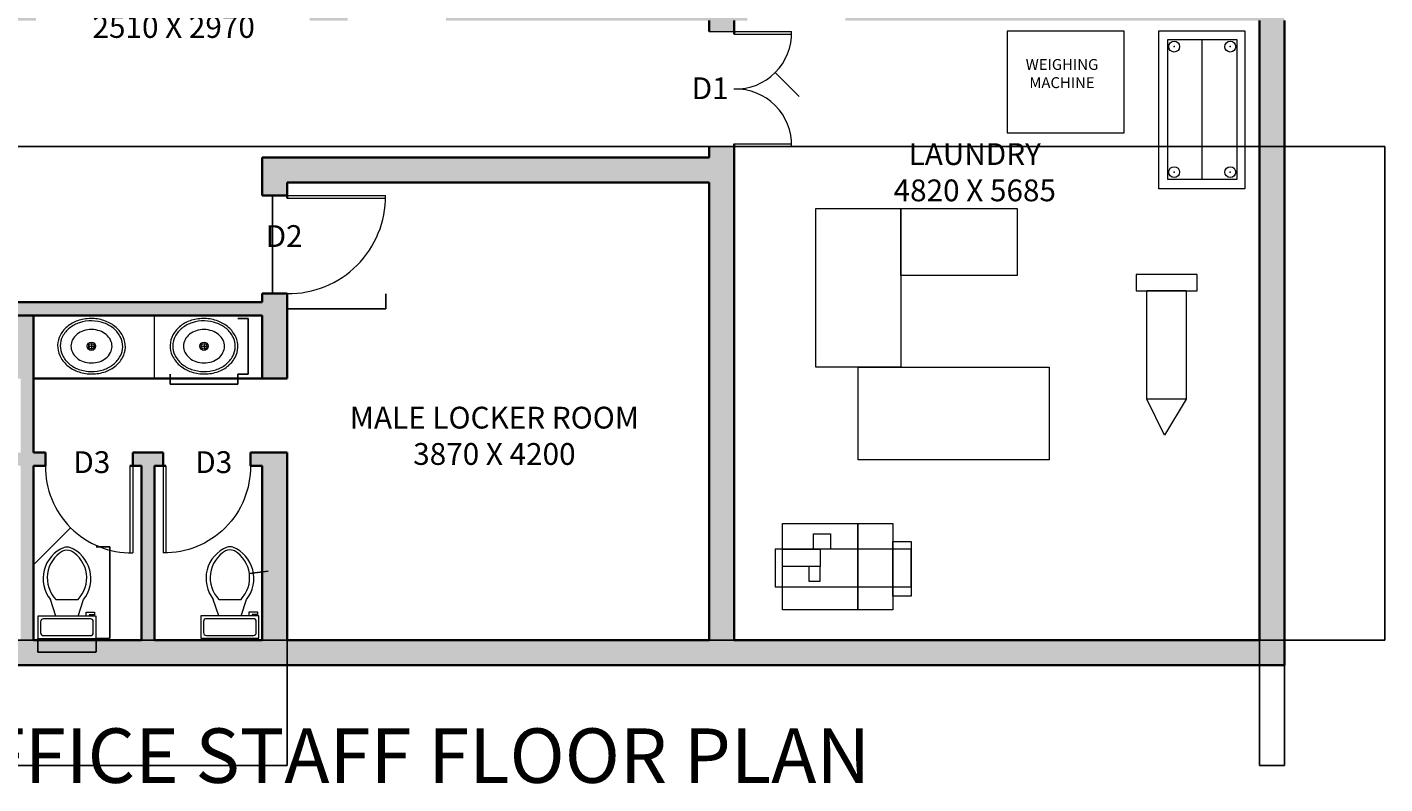
# Model space of a CAD drawing. Units: millimetres. Extents: x 14737 to 34075, y 1723 to 15415.
# Tile 2 of 2: x 21616 to 34075, y 1723 to 8669. Entities that reach past the tile are written whole.
import ezdxf

# ---------------------------------------------------------------- set-up
doc = ezdxf.new("R2010")
doc.units = ezdxf.units.MM
doc.header["$PDMODE"] = 32
doc.header["$PDSIZE"] = 100
for name, color, linetype, lineweight in [('A-ANNO-DIMS', 2, 'Continuous', 18), ('A-ANNO-TEXT', 7, 'Continuous', 18), ('A-ANNO-TITL', 7, 'Continuous', 35), ('A-AREA-IDEN', 7, 'Continuous', 25), ('A-DOOR', 4, 'Continuous', 18), ('A-DOOR-IDEN', 3, 'Continuous', 18), ('A-EQPM', 8, 'Continuous', 18), ('A-FLOR-FIXT', 9, 'Continuous', 18), ('A-WALL', 7, 'Continuous', 35), ('A-WALL-PATT', 252, 'Continuous', 13)]:
    doc.layers.add(name, color=color, linetype=linetype, lineweight=lineweight)
doc.styles.get("Standard").update_dxf_attribs({"font": 'arial.ttf'})
doc.dimstyles.get("Standard").update_dxf_attribs({"dimtxt": 0.18, "dimasz": 0.18, "dimexe": 0.18, "dimexo": 0.0625, "dimgap": 0.09, "dimtad": 0, "dimtih": 1, "dimtoh": 1, "dimdec": 4, "dimzin": 0, "dimdsep": 46, "dimtxsty": 'Standard', "dimcen": 0.09, "dimadec": 0, "dimazin": 0, "dimtfac": 1, "dimtdec": 4, "dimtofl": 0, "dimtmove": 0, "dimatfit": 3, "dimfxl": 1, "dimtolj": 1, "dimtzin": 0, "dimarcsym": 0})

# ---------------------------------------------------------------- blocks, each defined once
blk = doc.blocks.new('Sink - Oval top')
for p, q in [((-1, 0), (1, 0)), ((0, 1), (0, -1))]:
    blk.add_line(p, q)
for points in [[(-12.23371880354079, 0.3941914712607968, 0.1176342565883263), (-11.46456229543957, -3.361933235489118, 0.104469279667093), (-8.878748691070427, -6.803541973650567, 0.0900157896014849), (-5.082757700676665, -9.072309807490512, 0.0819199491592185), (-0.3227280122732736, -10.01585280257211, 0.0819199491592091), (4.488169920880977, -9.380701564817912, 0.0900157896014801), (8.422342359155778, -7.36101289847943, 0.1044692796670922), (11.22435122606941, -4.093009071543406, 0.1176342565883338), (12.23371880354091, -0.3941914712607968, 0.1176342565883057), (11.46456229543992, 3.361933235488777, 0.1044692796670849), (8.878748691070427, 6.803541973650567, 0.0900157896014884), (5.082757700676324, 9.072309807490681, 0.0819199491592058), (0.3227280122732736, 10.01585280257211, 0.081919949159207), (-4.488169920880864, 9.380701564817969, 0.0900157896014802), (-8.422342359155778, 7.36101289847943, 0.1044692796670951), (-11.22435122606919, 4.093009071543633, 0.1176342565883402)], [(-11.28627986850119, 0.1590597164737346, 0.1186217001864142), (-10.51590095791209, -3.253161772358112, 0.1046781721811095), (-8.071803350560115, -6.358618019863342, 0.0895620664691738), (-4.537699193222351, -8.366971929609804, 0.0811846988912177), (-0.1289739026695997, -9.15150355811437, 0.0811846988912276), (4.300109150126218, -8.491524865184601, 0.0895620664691798), (7.889406708212618, -6.583562428127606, 0.1046781721811044), (10.42004782883111, -3.548216131892445, 0.1186217001864013), (11.28627986850119, -0.1590597164736209, 0.1186217001863945), (10.51590095791221, 3.253161772357998, 0.1046781721811069), (8.071803350560115, 6.358618019863342, 0.0895620664691756), (4.537699193222124, 8.366971929609917, 0.081184698891216), (0.1289739026695997, 9.151503558114428, 0.0811846988912142), (-4.300109150125877, 8.491524865184829, 0.0895620664691747), (-7.889406708212618, 6.583562428127606, 0.1046781721811045), (-10.42004782883111, 3.548216131892445, 0.1186217001863946)], [(-7.420452389032902, 0.0829876781601797, 0.1182825673856775), (-6.907065465214486, -2.1674649380775, 0.1046074595377274), (-5.294791470712084, -4.209988192029413, 0.0897179636260996), (-2.966599981142508, -5.528122152688069, 0.0814360825277113), (-0.0675135187855176, -6.036810076758797, 0.0814360825277218), (2.84222437824053, -5.593085960977873, 0.0897179636261315), (5.199312936802016, -4.327350491993342, 0.1046074595376878), (6.85686365682659, -2.321395784920355, 0.1182825673856714), (7.420452389033016, -0.0829876781601797, 0.1182825673856961), (6.907065465214486, 2.167464938077614, 0.1046074595377135), (5.294791470712084, 4.209988192029413, 0.0897179636261265), (2.966599981142621, 5.528122152687842, 0.0814360825277426), (0.0675135187855176, 6.036810076758797, 0.0814360825277225), (-2.842224378240644, 5.593085960977873, 0.0897179636261212), (-5.199312936802016, 4.327350491993342, 0.1046074595377049), (-6.856863656826476, 2.321395784920355, 0.1182825673856712)]]:
    blk.add_lwpolyline(points, format="xyb", close=True)
for radius in [1.5, 1]:
    blk.add_circle((0, 0), radius)
blk = doc.blocks.new('Toilet - top')
for p, q in [((9.5, -6), (9.5, -2)), ((-10, -8.5), (-8, -8.5)), ((-10, -9.5), (-10, -8.5)), ((-7, -9.5), (-10, -9.5)), ((-8, -8.5), (-8, -8)), ((-7, -8), (-7, -9.5)), ((-4, -8), (-6, -14)), ((4, -8), (6, -14)), ((4, -14), (-4, -14))]:
    blk.add_line(p, q)
blk.add_lwpolyline([(10.5, -8), (10.5, 0), (-10.5, 0), (-10.5, -8)], close=True)
for points in [[(-9.5, -2), (-9.5, -6)], [(8.5, -1), (-8.5, -1)], [(-8.5, -7), (8.5, -7)]]:
    blk.add_lwpolyline(points)
for centre, radius, start, end in [((-8.625, -1.875), 0.8838834999999999, 81.86989999999999, 188.1301), ((8.625, -1.875), 0.8838834999999999, 351.8699, 98.13009999999998), ((-8.625, -6.125), 0.8838834999999999, 171.869898, 278.1301), ((8.625, -6.125), 0.8838834999999999, 261.8699, 8.130099999999993), ((3.519562435188956, -21.58049502388982), 12.16902005083646, 141.4691096810948, 247.9714346835576), ((4.199957580658807, -21.81740929088453), 11.3291791325804, 136.3677254423718, 238.946823937405), ((-3.519499936778316, -21.58047137067522), 12.16903423757823, 292.0284332733152, 38.53070636800453), ((-4.199890672038477, -21.81738596564128), 11.32918622148567, 301.0530065773863, 43.63209216694732), ((2.09660981727e-05, -27.87646475467881), 4, 245.7318247449371, 294.2681740488959), ((2.09415214183e-05, -28.99996806116075), 4, 254.8605283244437, 285.1394707718433)]:
    blk.add_arc(centre, radius, start, end)
blk = doc.blocks.new('DOOR-D2-900')
for p, q in [((-3.638e-12, 0), (-3.638e-12, 900)), ((25.39999999999782, 0), (25.39999999999782, 900))]:
    blk.add_line(p, q)
blk.add_arc((12.69999999999709, 12.69999999999891), 887.3908834330009, 359.1799766532175, 90.82002334678252)
blk = doc.blocks.new('DOOR-D3-800')
for p, q in [((774.702568529894, 800.102568529895), (774.702568529894, 0.1025685298941426)), ((800.1025685298955, 800.102568529895), (800.1025685298955, 0.1025685298941426))]:
    blk.add_line(p, q)
blk.add_arc((787.4025685298947, 787.4025685298961), 787.4024257011142, 179.0758372986705, 270.9241627013018)
blk = doc.blocks.new('*D10')
at = {"layer": 'A-ANNO-DIMS', "color": 0, "lineweight": -2, "transparency": 16777216}
for p, q in [((24003.52093727598, 7123.424739032067), (23867.88874532247, 7123.424739032067)), ((23868.06874532247, 7123.244739032067), (23868.06874532247, 6671.891063711406)), ((23868.06874532247, 6220.173459332084), (23868.06874532247, 6671.527134652743)), ((24003.52093727895, 6219.993459332084), (23867.88874532247, 6219.993459332084))]:
    blk.add_line(p, q, dxfattribs=at)
at = {"layer": 'A-ANNO-DIMS', "color": 0, "transparency": 16777216}
for points in [[(23868.03874532247, 7123.244739032067), (23868.09874532247, 7123.244739032067), (23868.06874532247, 7123.424739032067)], [(23868.03874532247, 6220.173459332084), (23868.09874532247, 6220.173459332084), (23868.06874532247, 6219.993459332084)]]:
    blk.add_solid(points, dxfattribs=at)
at = {"layer": 'Defpoints', "color": 0, "transparency": 16777216}
for p in [(24003.58343727598, 7123.424739032067), (23868.06874532247, 6219.993459332084), (24003.58343727895, 6219.993459332084)]:
    blk.add_point(p, dxfattribs=at)
at = {"layer": 'A-ANNO-DIMS', "color": 0, "transparency": 16777216, "insert": (23868.06874532247, 6671.709099182066), "char_height": 0.18, "attachment_point": 5}
blk.add_mtext('\\A1;D2 903 TYP.', dxfattribs=at)
blk = doc.blocks.new('*D11')
at = {"layer": 'A-ANNO-DIMS', "color": 0, "lineweight": -2, "transparency": 16777216}
for p, q in [((24003.58343727894, 6219.93095933208), (24003.58343727894, 6084.298767378567)), ((24907.01471697893, 6219.930959335052), (24907.01471697893, 6084.298767378567)), ((24003.76343727895, 6084.478767378567), (24454.70106212211, 6084.478767378567)), ((24906.83471697893, 6084.478767378567), (24455.89709213575, 6084.478767378567))]:
    blk.add_line(p, q, dxfattribs=at)
at = {"layer": 'A-ANNO-DIMS', "color": 0, "transparency": 16777216}
for points in [[(24003.76343727895, 6084.508767378568), (24003.76343727895, 6084.448767378567), (24003.58343727894, 6084.478767378567)], [(24906.83471697893, 6084.508767378568), (24906.83471697893, 6084.448767378567), (24907.01471697893, 6084.478767378567)]]:
    blk.add_solid(points, dxfattribs=at)
at = {"layer": 'Defpoints', "color": 0, "transparency": 16777216}
for p in [(24003.58343727894, 6219.99345933208), (24907.01471697893, 6219.993459335051), (24907.01471697893, 6084.478767378567)]:
    blk.add_point(p, dxfattribs=at)
at = {"layer": 'A-ANNO-DIMS', "color": 0, "transparency": 16777216, "insert": (24455.29907712893, 6084.478767378567), "char_height": 0.18, "attachment_point": 5}
blk.add_mtext('\\A1;903 TYP.', dxfattribs=at)
blk = doc.blocks.new('*D12')
at = {"layer": 'A-ANNO-DIMS', "color": 0, "lineweight": -2, "transparency": 16777216}
for p, q in [((22248.02062752452, 3898.382496057406), (22374.04431771571, 3898.382496057406)), ((22373.86431771571, 3898.202496057405), (22373.86431771571, 3478.878326388779)), ((22373.86431771571, 3059.187894782909), (22373.86431771571, 3478.512064451535)), ((22248.02062752452, 3059.007894782909), (22374.04431771571, 3059.007894782909))]:
    blk.add_line(p, q, dxfattribs=at)
at = {"layer": 'A-ANNO-DIMS', "color": 0, "transparency": 16777216}
for points in [[(22373.83431771571, 3898.202496057405), (22373.89431771571, 3898.202496057405), (22373.86431771571, 3898.382496057406)], [(22373.83431771571, 3059.187894782909), (22373.89431771571, 3059.187894782909), (22373.86431771571, 3059.007894782909)]]:
    blk.add_solid(points, dxfattribs=at)
at = {"layer": 'Defpoints', "color": 0, "transparency": 16777216}
for p in [(22247.95812752453, 3898.382496057406), (22247.95812752453, 3059.007894782909), (22373.86431771571, 3059.007894782909)]:
    blk.add_point(p, dxfattribs=at)
at = {"layer": 'A-ANNO-DIMS', "color": 0, "transparency": 16777216, "insert": (22373.86431771571, 3478.69519542015), "char_height": 0.18, "attachment_point": 5}
blk.add_mtext('\\A1;WC 839 TYP.', dxfattribs=at)
blk = doc.blocks.new('*D13')
at = {"layer": 'A-ANNO-DIMS', "color": 0, "lineweight": -2, "transparency": 16777216}
for p, q in [((21714.55812752452, 3058.945394782908), (21714.55812752452, 2932.921704591734)), ((22247.95812752452, 3058.945394782908), (22247.95812752452, 2932.921704591734)), ((21714.73812752452, 2933.101704591734), (21980.6601125177, 2933.101704591734)), ((22247.77812752452, 2933.101704591734), (21981.85614253134, 2933.101704591734))]:
    blk.add_line(p, q, dxfattribs=at)
at = {"layer": 'A-ANNO-DIMS', "color": 0, "transparency": 16777216}
for points in [[(21714.73812752452, 2933.131704591734), (21714.73812752452, 2933.071704591734), (21714.55812752452, 2933.101704591734)], [(22247.77812752452, 2933.131704591734), (22247.77812752452, 2933.071704591734), (22247.95812752452, 2933.101704591734)]]:
    blk.add_solid(points, dxfattribs=at)
at = {"layer": 'Defpoints', "color": 0, "transparency": 16777216}
for p in [(21714.55812752452, 3059.007894782908), (22247.95812752452, 3059.007894782908), (21714.55812752452, 2933.101704591734)]:
    blk.add_point(p, dxfattribs=at)
at = {"layer": 'A-ANNO-DIMS', "color": 0, "transparency": 16777216, "insert": (21981.25812752452, 2933.101704591734), "char_height": 0.18, "attachment_point": 5}
blk.add_mtext('\\A1;533 TYP.', dxfattribs=at)
blk = doc.blocks.new('*D16')
at = {"layer": 'A-ANNO-DIMS', "color": 0, "lineweight": -2, "transparency": 16777216}
for p, q in [((22927.15663479012, 5484.097901749652), (22927.15663479012, 5390.441495036614)), ((23550.74934621037, 5484.097901749652), (23550.74934621037, 5390.441495036614)), ((22927.33663479011, 5390.621495036614), (23237.94672174172, 5390.621495036614)), ((23550.56934621037, 5390.621495036614), (23239.95925925877, 5390.621495036614))]:
    blk.add_line(p, q, dxfattribs=at)
at = {"layer": 'A-ANNO-DIMS', "color": 0, "transparency": 16777216}
for points in [[(22927.33663479011, 5390.651495036614), (22927.33663479011, 5390.591495036614), (22927.15663479012, 5390.621495036614)], [(23550.56934621037, 5390.651495036614), (23550.56934621037, 5390.591495036614), (23550.74934621037, 5390.621495036614)]]:
    blk.add_solid(points, dxfattribs=at)
at = {"layer": 'Defpoints', "color": 0, "transparency": 16777216}
for p in [(22927.15663479012, 5484.160401749652), (23550.74934621037, 5484.160401749652), (23550.74934621037, 5390.621495036614)]:
    blk.add_point(p, dxfattribs=at)
at = {"layer": 'A-ANNO-DIMS', "color": 0, "transparency": 16777216, "insert": (23238.95299050024, 5390.621495036614), "char_height": 0.18, "attachment_point": 5}
blk.add_mtext('\\A1;BASIN 624 TYP.', dxfattribs=at)
blk = doc.blocks.new('*D17')
at = {"layer": 'A-ANNO-DIMS', "color": 0, "lineweight": -2, "transparency": 16777216}
for p, q in [((23550.81184621037, 5995.629815192883), (23644.46825292342, 5995.629815192883)), ((23644.28825292342, 5995.449815192883), (23644.28825292342, 5740.077011609059)), ((23644.28825292342, 5484.340401749654), (23644.28825292342, 5739.71320533348)), ((23550.81184621037, 5484.160401749654), (23644.46825292342, 5484.160401749654))]:
    blk.add_line(p, q, dxfattribs=at)
at = {"layer": 'A-ANNO-DIMS', "color": 0, "transparency": 16777216}
for points in [[(23644.25825292342, 5995.449815192883), (23644.31825292342, 5995.449815192883), (23644.28825292342, 5995.629815192883)], [(23644.25825292342, 5484.340401749654), (23644.31825292342, 5484.340401749654), (23644.28825292342, 5484.160401749654)]]:
    blk.add_solid(points, dxfattribs=at)
at = {"layer": 'Defpoints', "color": 0, "transparency": 16777216}
for p in [(23550.74934621038, 5995.629815192883), (23644.28825292342, 5995.629815192883), (23550.74934621038, 5484.160401749654)]:
    blk.add_point(p, dxfattribs=at)
at = {"layer": 'A-ANNO-DIMS', "color": 0, "transparency": 16777216, "insert": (23644.28825292342, 5739.895108471261), "char_height": 0.18, "attachment_point": 5}
blk.add_mtext('\\A1;511 TYP.', dxfattribs=at)
blk = doc.blocks.new('*D29')
at = {"layer": 'A-ANNO-DIMS', "color": 0, "lineweight": -2, "transparency": 16777216}
for p, q in [((19338.583437, 3043.362239), (19338.583437, 1892.244739)), ((24003.583437, 3043.362239), (24003.583437, 1892.244739)), ((19338.763437, 1892.424739), (21670.72036742292, 1892.424739)), ((24003.403437, 1892.424739), (21671.44650657708, 1892.424739))]:
    blk.add_line(p, q, dxfattribs=at)
at = {"layer": 'A-ANNO-DIMS', "color": 0, "transparency": 16777216}
for points in [[(19338.763437, 1892.454739), (19338.763437, 1892.394739), (19338.583437, 1892.424739)], [(24003.403437, 1892.454739), (24003.403437, 1892.394739), (24003.583437, 1892.424739)]]:
    blk.add_solid(points, dxfattribs=at)
at = {"layer": 'Defpoints', "color": 0, "transparency": 16777216}
for p in [(19338.583437, 3043.424739), (24003.583437, 3043.424739), (24003.583437, 1892.424739)]:
    blk.add_point(p, dxfattribs=at)
at = {"layer": 'A-ANNO-DIMS', "color": 0, "transparency": 16777216, "insert": (21671.083437, 1892.424739), "char_height": 0.18, "attachment_point": 5}
blk.add_mtext('\\A1;4665', dxfattribs=at)
blk = doc.blocks.new('*D31')
at = {"layer": 'A-ANNO-DIMS', "color": 0, "lineweight": -2, "transparency": 16777216}
for p, q in [((15888.64593700001, 7573.424739000003), (34074.76343700003, 7573.424739000007)), ((34074.58343700003, 7573.244739000006), (34074.58343700003, 5308.606703529336)), ((34074.58343700003, 3043.604739000004), (34074.58343700003, 5308.242774470673)), ((15888.64593700001, 3043.424739000001), (34074.76343700003, 3043.424739000004))]:
    blk.add_line(p, q, dxfattribs=at)
at = {"layer": 'A-ANNO-DIMS', "color": 0, "transparency": 16777216}
for points in [[(34074.55343700003, 7573.244739000006), (34074.61343700003, 7573.244739000006), (34074.58343700003, 7573.424739000007)], [(34074.55343700003, 3043.604739000004), (34074.61343700003, 3043.604739000004), (34074.58343700003, 3043.424739000004)]]:
    blk.add_solid(points, dxfattribs=at)
at = {"layer": 'Defpoints', "color": 0, "transparency": 16777216}
for p in [(15888.58343700001, 7573.424739000003), (34074.58343700003, 7573.424739000007), (15888.58343700001, 3043.424739000001)]:
    blk.add_point(p, dxfattribs=at)
at = {"layer": 'A-ANNO-DIMS', "color": 0, "transparency": 16777216, "insert": (34074.58343700002, 5308.424738999995), "char_height": 0.18, "attachment_point": 5}
blk.add_mtext('\\A1;4530', dxfattribs=at)
blk = doc.blocks.new('*D32')
at = {"layer": 'A-ANNO-DIMS', "color": 0, "lineweight": -2, "transparency": 16777216}
for p, q in [((32923.583437, 3043.362239), (32923.583437, 1892.244739)), ((33153.583437, 2813.362239), (33153.583437, 1892.244739)), ((32923.763437, 1892.424739), (33038.2933619659, 1892.424739)), ((33153.403437, 1892.424739), (33038.87351203411, 1892.424739))]:
    blk.add_line(p, q, dxfattribs=at)
at = {"layer": 'A-ANNO-DIMS', "color": 0, "transparency": 16777216}
for points in [[(32923.763437, 1892.454739), (32923.763437, 1892.394739), (32923.583437, 1892.424739)], [(33153.403437, 1892.454739), (33153.403437, 1892.394739), (33153.583437, 1892.424739)]]:
    blk.add_solid(points, dxfattribs=at)
at = {"layer": 'Defpoints', "color": 0, "transparency": 16777216}
for p in [(32923.583437, 3043.424739), (33153.583437, 2813.424739), (33153.583437, 1892.424739)]:
    blk.add_point(p, dxfattribs=at)
at = {"layer": 'A-ANNO-DIMS', "color": 0, "transparency": 16777216, "insert": (33038.583437, 1892.424739), "char_height": 0.18, "attachment_point": 5}
blk.add_mtext('\\A1;230', dxfattribs=at)
blk = doc.blocks.new('*D35')
at = {"layer": 'A-ANNO-DIMS', "color": 0, "lineweight": -2, "transparency": 16777216}
for p, q in [((22571.79343699999, 4630.724738999999), (22571.97343699999, 4630.724738999999)), ((22571.883437, 4630.634738999997), (22571.883437, 4630.814738999998)), ((21681.03952663161, 3739.88034543161), (22014.9787138139, 4073.819713744867)), ((21680.85952663161, 3739.88034543161), (21681.03952663161, 3739.88034543161))]:
    blk.add_line(p, q, dxfattribs=at)
at = {"layer": 'A-ANNO-DIMS', "color": 0, "transparency": 16777216}
blk.add_solid([(22014.95750060472, 4073.84092694255), (22014.99992702309, 4073.798500547183), (22015.105993, 4073.946992999999)], dxfattribs=at)
at = {"layer": 'Defpoints', "color": 0, "transparency": 16777216}
for p in [(22571.883437, 4630.724738999999), (22015.105993, 4073.946992999999)]:
    blk.add_point(p, dxfattribs=at)
at = {"layer": 'A-ANNO-DIMS', "color": 0, "transparency": 16777216, "insert": (21680.18305323461, 3739.880345431608), "char_height": 0.18, "attachment_point": 5}
blk.add_mtext('\\A1;4X R787.4', dxfattribs=at)
blk = doc.blocks.new('*D36')
at = {"layer": 'A-ANNO-DIMS', "color": 0, "lineweight": -2, "transparency": 16777216}
for p, q in [((28116.193437, 8615.724739), (28116.373437, 8615.724739)), ((28116.283437, 8615.634738999997), (28116.283437, 8615.814739)), ((28698.89021582972, 8033.117678570288), (28480.53995318986, 8251.468046748627)), ((28699.07021582972, 8033.117678570288), (28698.89021582972, 8033.117678570288))]:
    blk.add_line(p, q, dxfattribs=at)
at = {"layer": 'A-ANNO-DIMS', "color": 0, "transparency": 16777216}
blk.add_solid([(28480.56116639842, 8251.489259946937), (28480.51873998129, 8251.44683355032), (28480.412674, 8251.595326)], dxfattribs=at)
at = {"layer": 'Defpoints', "color": 0, "transparency": 16777216}
for p in [(28116.28343699999, 8615.724739), (28480.412674, 8251.595326)]:
    blk.add_point(p, dxfattribs=at)
at = {"layer": 'A-ANNO-DIMS', "color": 0, "transparency": 16777216, "insert": (28699.64287612986, 8033.117678570286), "char_height": 0.18, "attachment_point": 5}
blk.add_mtext('\\A1;4X R515', dxfattribs=at)
blk = doc.blocks.new('*D38')
at = {"layer": 'A-ANNO-DIMS', "color": 0, "lineweight": -2, "transparency": 16777216}
for p, q in [((23370.12200999999, 3615.312254999999), (23370.30200999999, 3615.312254999999)), ((23370.21201, 3615.222254999999), (23370.21200999999, 3615.402254999999)), ((23826.52884221145, 3676.627307828413), (23655.5884267143, 3653.658134072706))]:
    blk.add_line(p, q, dxfattribs=at)
at = {"layer": 'A-ANNO-DIMS', "color": 0, "transparency": 16777216}
blk.add_solid([(23655.58443153552, 3653.687866858422), (23655.59242189309, 3653.628401286989), (23655.41003, 3653.634162999999)], dxfattribs=at)
at = {"layer": 'Defpoints', "color": 0, "transparency": 16777216}
for p in [(23370.21201, 3615.312254999999), (23655.41003, 3653.634162999999)]:
    blk.add_point(p, dxfattribs=at)
at = {"layer": 'A-ANNO-DIMS', "color": 0, "transparency": 16777216, "insert": (23827.27204821418, 3676.627307828413), "char_height": 0.18, "attachment_point": 5}
blk.add_mtext('\\A1;8X R287.76', dxfattribs=at)

msp = doc.modelspace()

# ---------------------------------------------------------------- hatches: boundary and pattern name
at = {"layer": 'A-WALL-PATT'}
h = msp.add_hatch(color=256, dxfattribs=at)
h.dxf.hatch_style = 1
h.paths.add_polyline_path([(15888.58343727589, 14263.42473903341), (21468.58343727589, 14263.42473903341), (21468.58343727589, 8848.424739033417), (17848.13203580986, 8848.424739033413), (17848.13203580986, 8728.424739033415), (21698.58343727589, 8728.424739033415), (21698.58343727589, 14493.42473903341), (15658.58343727589, 14493.42473903341), (15658.58343727589, 8728.424739033415), (15658.58343727589, 8628.424739033413), (15888.58343727588, 8628.424739033413), (15888.58343727588, 8728.424739033415), (16948.13203580987, 8728.424739033415), (16948.13203580987, 8848.424739033413), (15888.58343727589, 8848.424739033413)])
h.paths.add_polyline_path([(33153.58343727589, 13323.42473903341), (27983.58343727589, 13323.42473903341), (24480.16591345426, 13323.42473903341), (24480.16591345426, 13093.42473903341), (27983.58343727589, 13093.42473903341), (27983.58343727589, 11423.42473903341), (23613.58343727589, 11423.42473903341), (23613.58343727589, 13323.42473903341), (23493.58343727589, 13323.42473903341), (23493.58343727589, 11303.42473903341), (24208.58343727589, 11303.42473903341), (24208.58343727589, 9367.011203696671), (24208.58343727589, 8728.424739033415), (24558.5834372759, 8728.424739033411), (24558.5834372759, 8848.424739033413), (24438.5834372759, 8848.424739033413), (24438.5834372759, 11303.42473903341), (27983.58343727589, 11303.42473903341), (27983.58343727589, 8848.42473903341), (25458.58343727589, 8848.424739033413), (25458.58343727589, 8728.424739033411), (27873.58343727589, 8728.42473903341), (27873.58343727589, 8628.424739033413), (28103.58343727589, 8628.424739033413), (28103.58343727589, 8728.42473903341), (28223.58343727589, 8728.42473903341), (28223.58343727589, 8848.424739033408), (28103.58343727589, 8848.42473903341), (28103.58343727589, 13093.42473903341), (32923.58343727589, 13093.42473903341), (32923.5834372759, 8848.42473903341), (29123.58343727589, 8848.424739033408), (29123.58343727589, 8728.42473903341), (32923.58343727589, 8728.42473903341), (32923.58343727589, 3043.424739033409), (28103.58343727589, 3043.424739033409), (28103.58343727589, 7573.424739033412), (27873.58343727589, 7573.424739033412), (27873.58343727589, 7473.424739033409), (23773.5834372759, 7473.424739033409), (23773.58343727589, 7123.424739033409), (24003.5834372759, 7123.424739033409), (24003.5834372759, 7243.424739033409), (27873.58343727589, 7243.424739033409), (27873.58343727589, 3043.424739033409), (24003.58343727589, 3043.42473903341), (24003.58343727589, 4763.42473903341), (23664.58343727588, 4763.42473903341), (23664.58343727588, 4643.424739033411), (23773.58343727589, 4643.42473903341), (23773.58343727589, 3043.424739033409), (22784.58343727589, 3043.424739033409), (22784.58343727588, 4643.42473903341), (22864.58343727588, 4643.424739033411), (22864.58343727588, 4763.424739033409), (22584.58343727588, 4763.424739033409), (22584.58343727588, 4643.424739033409), (22664.58343727588, 4643.424739033409), (22664.58343727589, 3043.424739033409), (21675.58343727589, 3043.424739033409), (21675.58343727589, 4643.424739033409), (21784.58343727588, 4643.424739033409), (21784.58343727588, 4763.424739033409), (21675.58343727589, 4763.42473903341), (21675.58343727589, 6023.424739033409), (19458.58343727589, 6023.424739033409), (19458.58343727589, 5443.424739033409), (21556.58343727589, 5443.424739033409), (21556.58343727589, 4763.424739033409), (21447.58343727589, 4763.42473903341), (21447.58343727589, 4643.424739033409), (21556.58343727589, 4643.42473903341), (21556.58343727588, 3043.42473903341), (20567.58343727589, 3043.424739033409), (20567.58343727589, 4643.424739033409), (20647.58343727589, 4643.424739033409), (20647.58343727589, 4763.42473903341), (20367.58343727589, 4763.42473903341), (20367.58343727589, 4643.424739033409), (20447.58343727589, 4643.424739033409), (20447.58343727589, 3043.424739033409), (19458.58343727589, 3043.424739033409), (19458.58343727589, 4643.424739033409), (19567.58343727589, 4643.424739033409), (19567.58343727589, 4763.42473903341), (19338.58343727589, 4763.42473903341), (19338.58343727589, 3043.42473903341), (15888.58343727589, 3043.42473903341), (15888.58343727589, 7243.424739033411), (19338.58343727589, 7243.424739033411), (19338.58343727589, 7123.42473903341), (19458.58343727589, 7123.42473903341), (19458.58343727589, 7473.424739033409), (15888.58343727589, 7473.424739033411), (15888.58343727588, 7573.424739033412), (15658.58343727589, 7573.424739033412), (15658.58343727589, 7473.42473903341), (15658.58343727589, 2813.42473903341), (23773.58343727589, 2813.42473903341), (27873.58343727589, 2813.42473903341), (33153.58343727589, 2813.42473903341), (33153.58343727589, 8728.42473903341)])
h.paths.add_polyline_path([(24003.5834372759, 6223.424739033411), (23773.58343727589, 6223.424739033411), (23773.58343727589, 6143.42473903341), (19458.58343727589, 6143.42473903341), (19458.58343727589, 6223.42473903341), (19338.58343727589, 6223.424739033411), (19338.58343727589, 5443.42473903341), (19458.58343727589, 5443.42473903341), (19458.58343727589, 6023.424739033409), (21675.58343727589, 6023.424739033409), (23773.58343727589, 6023.424739033409), (23773.58343727589, 5443.42473903341), (24003.5834372759, 5443.42473903341)], flags=17)

# ---------------------------------------------------------------- linework, layer by layer
at = {"layer": 'A-DOOR'}
for p, q in [((27873.5834372759, 8628.424739033413), (28631.08343727589, 8628.424739033413)), ((28103.58343727589, 8603.024739033413), (28631.08343727589, 8603.024739033413)), ((28103.58343727589, 8100.611480549963), (28103.58343727589, 8100.924739033414)), ((27873.58343727589, 7573.424739033412), (28631.08343727589, 7573.424739033412)), ((28103.58343727589, 7598.82473903341), (28631.08343727589, 7598.82473903341))]:
    msp.add_line(p, q, dxfattribs=at)
for centre, start, end in [((28116.28343727589, 8615.724739033414), 268.586812670943, 1.413187329071083), ((28116.28343727589, 7585.811480549961), 358.586812670943, 91.41318732905698)]:
    msp.add_arc(centre, 514.9566292417265, start, end, dxfattribs=at)
at = {"layer": 'A-EQPM'}
for p, q in [((32398.7244555807, 7271.716835053656), (32398.7244555807, 8556.039657402518)), ((32053.8599697879, 4922.261864324373), (31891.82518392905, 5253.956048876967)), ((32250.97145432941, 5253.956048876967), (32053.8599697879, 4922.261864324373))]:
    msp.add_line(p, q, dxfattribs=at)
for points in [[(31683.8815333972, 8632.358277696558), (30608.31329569307, 8632.358277696558), (30608.31329569307, 7698.089827207038), (31683.8815333972, 7698.089827207038)], [(31999.88321656956, 8634.466678702587), (32790.01649717954, 8634.466678702587), (32790.01649717954, 7184.136033166277), (31999.88321656956, 7184.136033166277)], [(32082.29016317428, 8556.039657402518), (32715.15874798713, 8556.039657402518), (32715.15874798713, 7271.716835053656), (32082.29016317428, 7271.716835053656)], [(28852.7463469712, 7003.908936387809), (29632.14359201778, 7003.908936387809), (29632.14359201778, 5548.007278359532), (28852.7463469712, 5548.007278359532)], [(29632.14359201778, 7003.908936387809), (30699.91790528412, 7003.908936387809), (30699.91790528412, 6388.848886519561), (29632.14359201778, 6388.848886519561)], [(31793.21806810486, 6247.735490771727), (32353.99302419193, 6247.735490771727), (32353.99302419193, 6397.640227042768), (31793.21806810486, 6397.640227042768)], [(31891.82518392905, 6250.509042789734), (32250.97145432941, 6250.509042789734), (32250.97145432941, 5253.956048876967), (31891.82518392905, 5253.956048876967)], [(29242.44496949449, 5548.007278359532), (30993.95950792815, 5548.007278359532), (30993.95950792815, 4695.886375549169), (29242.44496949449, 4695.886375549169)], [(28548.19381132021, 4113.676854592472), (29239.73075695709, 4113.676854592472), (29239.73075695709, 3320.545975867259), (28548.19381132021, 3320.545975867259)], [(29239.73075695709, 4113.676854592472), (29559.88673147901, 4113.676854592472), (29559.88673147901, 3320.545975867259), (29239.73075695709, 3320.545975867259)], [(28987.78163331908, 3875.888953505939), (28830.63148671985, 3875.888953505939), (28830.63148671985, 4017.67797237328), (28987.78163331908, 4017.67797237328)], [(29727.90801905687, 3875.888953505939), (28480.84576583091, 3875.888953505939), (28480.84576583091, 3531.544185629646), (29727.90801905687, 3531.544185629646)], [(28548.19381132021, 3875.888953505939), (28893.96228413865, 3875.888953505939), (28893.96228413865, 3717.111415229865), (28548.19381132021, 3717.111415229865)], [(29559.88673147901, 3946.7834493423), (29727.90801905687, 3946.7834493423), (29727.90801905687, 3445.457986861919), (29559.88673147901, 3445.457986861919)], [(28893.96228413865, 3717.111415229865), (28790.07665573093, 3717.111415229865), (28790.07665573093, 3582.183122881885), (28893.96228413865, 3582.183122881885)]]:
    msp.add_lwpolyline(points, close=True, dxfattribs=at)
for p in [(32141.52340428181, 8489.987239589009), (32655.92550687961, 8489.987239589009), (32141.52340428181, 7337.769252867166), (32655.92550687961, 7337.769252867166)]:
    msp.add_point(p, dxfattribs=at)
at = {"layer": 'A-FLOR-FIXT'}
msp.add_line((22784.58343727589, 5443.424739033409), (22784.58343727589, 6023.424739033409), dxfattribs=at)
at = {"layer": 'A-WALL'}
for p, q in [((27873.5834372759, 8628.424739033413), (27873.58343727589, 8728.42473903341)), ((28103.58343727589, 8603.024739033413), (28103.58343727589, 8728.42473903341)), ((32923.58343727589, 3043.424739033409), (32923.58343727589, 8728.42473903341)), ((33153.58343727589, 2813.42473903341), (33153.58343727589, 8728.42473903341)), ((27873.58343727589, 7473.424739033409), (27873.58343727589, 7573.424739033412)), ((28103.58343727589, 3043.424739033409), (28103.58343727589, 7598.82473903341)), ((27873.58343727589, 7473.424739033409), (23773.58343727589, 7473.424739033409)), ((23773.58343727589, 7123.42473903341), (23773.5834372759, 7473.424739033409)), ((27873.58343727589, 7243.424739033409), (24003.58343727589, 7243.424739033409)), ((24003.5834372759, 7098.024739033409), (24003.5834372759, 7243.424739033409)), ((27873.58343727589, 3043.424739033409), (27873.5834372759, 7243.424739033409)), ((24003.5834372759, 7123.424739033409), (23773.5834372759, 7123.42473903341)), ((23773.58343727589, 6143.42473903341), (19458.58343727589, 6143.42473903341)), ((23773.58343727589, 6143.42473903341), (23773.58343727589, 6223.42473903341)), ((24003.5834372759, 6223.42473903341), (23773.5834372759, 6223.42473903341)), ((24003.5834372759, 5443.42473903341), (24003.5834372759, 6223.42473903341)), ((23773.58343727589, 6023.424739033409), (19458.58343727589, 6023.424739033409)), ((21675.58343727589, 4763.424739033409), (21675.58343727589, 6023.424739033409)), ((23773.58343727589, 5443.42473903341), (23773.58343727589, 6023.424739033409)), ((24003.58343727589, 5443.42473903341), (21675.58343727589, 5443.42473903341)), ((21784.58343727589, 4763.424739033409), (21675.58343727589, 4763.42473903341)), ((21784.58343727588, 4643.424739033409), (21784.58343727588, 4763.42473903341)), ((22584.58343727588, 4643.424739033409), (22584.58343727588, 4763.42473903341)), ((22864.58343727588, 4763.424739033409), (22584.58343727588, 4763.424739033409)), ((22864.58343727588, 4643.424739033409), (22864.58343727588, 4763.42473903341)), ((24003.58343727589, 4763.42473903341), (23664.58343727588, 4763.42473903341)), ((23664.58343727588, 4643.424739033409), (23664.58343727588, 4763.42473903341)), ((24003.58343727589, 3043.424739033409), (24003.58343727589, 4763.42473903341)), ((21675.58343727589, 3043.424739033413), (21675.58343727589, 4643.424739033409)), ((21784.58343727588, 4643.424739033409), (21675.58343727589, 4643.424739033409)), ((22664.58343727588, 4643.424739033409), (22559.18343727588, 4643.424739033409)), ((22664.58343727589, 3043.424739033412), (22664.58343727588, 4643.424739033409)), ((22784.58343727589, 3043.424739033412), (22784.58343727588, 4643.424739033409)), ((22889.98343727588, 4643.42473903341), (22784.58343727588, 4643.424739033409)), ((23773.5834372759, 4643.42473903341), (23664.58343727588, 4643.42473903341)), ((23773.58343727589, 3043.424739033409), (23773.58343727589, 4643.42473903341)), ((22664.58343727588, 3043.42473903341), (21675.58343727589, 3043.42473903341)), ((23773.58343727589, 3043.424739033409), (22784.58343727589, 3043.42473903341)), ((27873.58343727589, 3043.424739033409), (24003.58343727589, 3043.424739033409)), ((28103.58343727589, 3043.42473903341), (32923.58343727589, 3043.424739033409)), ((23773.58343727589, 2813.42473903341), (15658.58343727589, 2813.42473903341)), ((27873.58343727589, 2813.42473903341), (23773.58343727589, 2813.42473903341)), ((27873.58343727589, 2813.42473903341), (33153.58343727589, 2813.42473903341))]:
    msp.add_line(p, q, dxfattribs=at)

# ---------------------------------------------------------------- block references
at = {"layer": 'A-DOOR', "rotation": 270.0000000001885}
msp.add_blockref('DOOR-D2-900', (24003.58343727597, 7123.42473903206), dxfattribs=at)
at = {"layer": 'A-DOOR'}
msp.add_blockref('DOOR-D3-800', (21784.48086874601, 3843.322170503509), dxfattribs=at)
at = {"layer": 'A-DOOR', "extrusion": (0, 0, -1), "zscale": -1}
msp.add_blockref('DOOR-D3-800', (-23664.68600580581, 3843.322170503542), dxfattribs=at)
at = {"layer": 'A-FLOR-FIXT', "xscale": 25.4, "yscale": 25.4, "zscale": 25.4}
for p in [(22206.3966186125, 5739.895285812344), (23238.95299050024, 5739.895108471266)]:
    msp.add_blockref('Sink - Oval top', p, dxfattribs=at)
at = {"layer": 'A-FLOR-FIXT', "xscale": 25.4, "yscale": 25.4, "zscale": 25.4, "rotation": 180}
for p in [(21981.25812752452, 3059.007894782908), (23476.89093228709, 3061.150059510814)]:
    msp.add_blockref('Toilet - top', p, dxfattribs=at)

# ---------------------------------------------------------------- texts
at = {"layer": 'A-ANNO-TEXT', "insert": (29196.76552270493, 8375.929964000374), "char_height": 100, "attachment_point": 1}
msp.add_mtext_dynamic_manual_height_columns('\\pxqc;{\\fArial|b1|i0|c0|p34; WEIGHING\\P MACHINE}', width=3800.236613510075, gutter_width=12.5, heights=[0], dxfattribs=at)
at = {"layer": 'A-ANNO-TITL', "insert": (20711.77164831711, 2232.309858371271), "char_height": 500, "attachment_point": 1}
msp.add_mtext_dynamic_manual_height_columns('{\\fArial|b1|i0|c0|p34;OFFICE STAFF FLOOR PLAN}', width=11408.76462508039, gutter_width=12.5, heights=[0], dxfattribs=at)
at = {"layer": 'A-AREA-IDEN', "char_height": 200, "attachment_point": 1}
for s, insert in [('\\pxqc;{\\fArial|b1|i0|c0|p34;RECEVING AREA\\P2510 X 2970}', (21060.59741427377, 9103.498921946622)), ('\\pxqc;{\\fArial|b1|i0|c0|p34;LAUNDRY\\P4820 X 5685}', (28411.71690961859, 7603.726305596747)), ('\\pxqc;{\\fArial|b1|i0|c0|p34;MALE LOCKER ROOM\\P3870 X 4200}', (24003.58343727589, 5184.534334303989))]:
    msp.add_mtext_dynamic_manual_height_columns(s, width=3800.236613510075, gutter_width=12.5, heights=[0], dxfattribs=dict(at, insert=insert))
at = {"layer": 'A-DOOR-IDEN', "char_height": 200, "attachment_point": 1}
for s, insert in [('D1', (27714.23639271641, 8207.66793817468)), ('D2', (23804.73511886644, 6850.90126322758)), ('D3', (22039.92749038199, 4776.022181917107)), ('D3', (23158.7469414114, 4776.022181917107))]:
    msp.add_mtext_dynamic_manual_height_columns(s, width=370.9848257368431, gutter_width=12.5, heights=[0], dxfattribs=dict(at, insert=insert))

# ---------------------------------------------------------------- dimensions: what is measured, and where the dimension line sits
at = {"layer": 'A-ANNO-DIMS'}
for center, mpoint, text, override, picture, middle in [((28116.28343699999, 8615.724739), (28480.412674, 8251.595326), '4X <>', {"dimdec": 0, "dimlfac": 1, "dimrnd": 0, "dimzin": 0, "dimdsep": 46, "dimlunit": 2}, '*D36', (28699.64287612986, 8033.117678570286)), ((22571.883437, 4630.724738999999), (22015.105993, 4073.946992999999), '4X <>', {"dimdec": 1, "dimlfac": 1, "dimrnd": 0, "dimzin": 0, "dimdsep": 46, "dimlunit": 2}, '*D35', (21680.18305323461, 3739.880345431608)), ((23370.21201, 3615.312254999999), (23655.41003, 3653.634162999999), '8X <>', {"dimdec": 2, "dimlfac": 1, "dimrnd": 0, "dimzin": 0, "dimdsep": 46, "dimlunit": 2}, '*D38', (23826.52884221145, 3676.627307828414))]:
    dim = msp.add_radius_dim(center=center, mpoint=mpoint, text=text, dimstyle='Standard', override=override, dxfattribs=at)
    dim.commit()
    dim.dimension.update_dxf_attribs({"geometry": picture, "text_midpoint": middle, "dimtype": 164})
dim = msp.add_linear_dim(base=(34074.58343700003, 7573.424739000007), p1=(15888.583437, 3043.424739), p2=(15888.583437, 7573.424739), angle=90, dimstyle='Standard', override={"dimdec": 0, "dimlfac": 1, "dimrnd": 0, "dimzin": 0, "dimdsep": 46, "dimlunit": 2}, dxfattribs=at)
dim.commit()
dim.dimension.update_dxf_attribs({"geometry": '*D31', "text_midpoint": (34074.58343700002, 5308.424738999995)})
for base, p1, p2, angle, text, picture, middle in [((23868.06874532247, 6219.993459332084), (24003.58343727597, 7123.424739032063), (24003.58343727894, 6219.99345933208), 270.0000000001885, 'D2 <> TYP.', '*D10', (23868.06874532247, 6671.709099182066)), ((24907.01471697893, 6084.478767378567), (24003.58343727894, 6219.99345933208), (24907.01471697893, 6219.993459335051), 1.884416e-10, '<> TYP.', '*D11', (24455.29907712893, 6084.478767378567)), ((23644.28825292342, 5995.629815192883), (23550.74934621037, 5484.160401749652), (23550.74934621037, 5995.629815192881), 90, '<> TYP.', '*D17', (23644.28825292342, 5739.895108471261)), ((22373.86431771571, 3059.007894782909), (22247.95812752452, 3898.382496057403), (22247.95812752452, 3059.007894782908), 270, 'WC <> TYP.', '*D12', (22373.86431771571, 3478.69519542015)), ((21714.55812752452, 2933.101704591734), (22247.95812752452, 3059.007894782908), (21714.55812752452, 3059.007894782908), 180, '<> TYP.', '*D13', (21981.25812752452, 2933.101704591734))]:
    dim = msp.add_linear_dim(base=base, p1=p1, p2=p2, angle=angle, text=text, dimstyle='Standard', override={"dimdec": 0, "dimlfac": 1, "dimrnd": 0, "dimzin": 0, "dimdsep": 46, "dimlunit": 2}, dxfattribs=at)
    dim.commit()
    dim.dimension.update_dxf_attribs({"geometry": picture, "text_midpoint": middle})
dim = msp.add_linear_dim(base=(23550.74934621037, 5390.621495036614), p1=(22927.15663479012, 5484.160401749652), p2=(23550.74934621037, 5484.160401749652), text='BASIN <> TYP.', dimstyle='Standard', override={"dimdec": 0, "dimlfac": 1, "dimrnd": 0, "dimzin": 0, "dimdsep": 46, "dimlunit": 2}, dxfattribs=at)
dim.commit()
dim.dimension.update_dxf_attribs({"geometry": '*D16', "text_midpoint": (23238.95299050024, 5390.621495036614)})
for base, p1, p2, picture, middle in [((24003.583437, 1892.424739), (19338.583437, 3043.424739), (24003.583437, 3043.424739), '*D29', (21671.083437, 1892.424739)), ((33153.583437, 1892.424739), (32923.583437, 3043.424739), (33153.583437, 2813.424739), '*D32', (33038.583437, 1892.424739))]:
    dim = msp.add_linear_dim(base=base, p1=p1, p2=p2, dimstyle='Standard', override={"dimdec": 0, "dimlfac": 1, "dimrnd": 0, "dimzin": 0, "dimdsep": 46, "dimlunit": 2}, dxfattribs=at)
    dim.commit()
    dim.dimension.update_dxf_attribs({"geometry": picture, "text_midpoint": middle})

doc.saveas('drawing.dxf')
